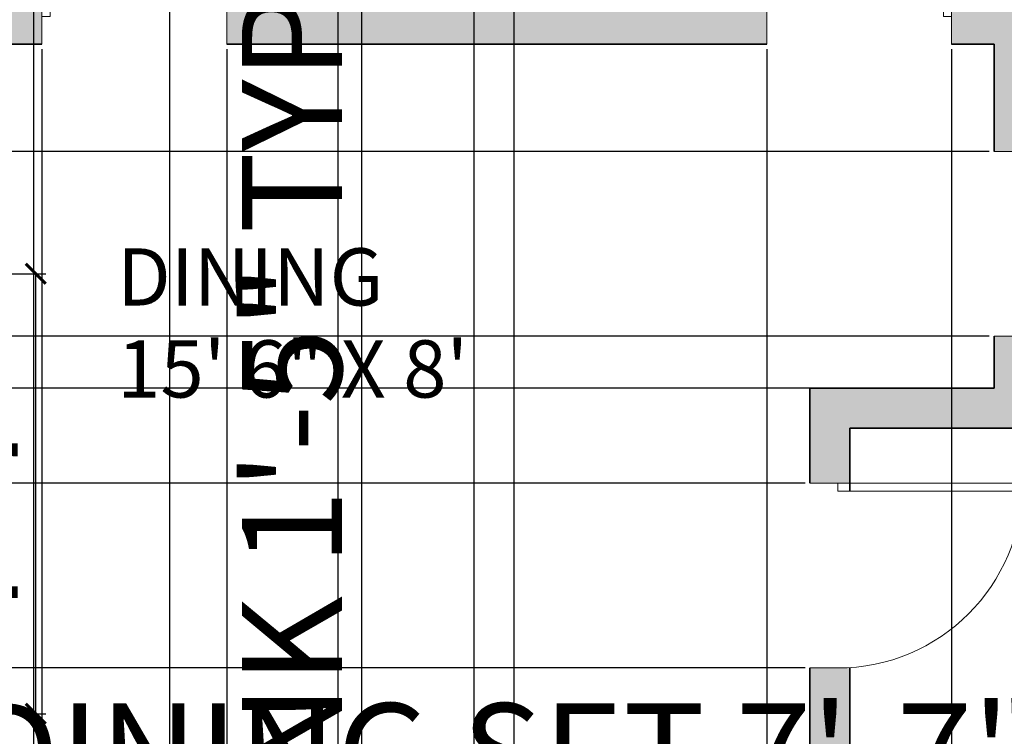
# Model space of a CAD drawing. Units: inches. Extents: x 1763 to 2368, y 1500 to 2097.
# Tile 10 of 24: x 1956 to 2079, y 1794 to 1883. Entities that reach past the tile are written whole.
import ezdxf

# ---------------------------------------------------------------- set-up
doc = ezdxf.new("R2010")
doc.units = ezdxf.units.IN
for name, color, linetype, lineweight in [('A-ANNO-DIMS', 2, 'Continuous', 18), ('A-AREA-IDEN', 7, 'Continuous', 18), ('A-DOOR', 4, 'Continuous', 18), ('A-WALL', 7, 'Continuous', 35), ('A-WALL-PATT', 7, 'Continuous', 13)]:
    doc.layers.add(name, color=color, linetype=linetype, lineweight=lineweight)
doc.styles.get("Standard").update_dxf_attribs({"font": 'arial.ttf'})
doc.dimstyles.new('ISO-25', dxfattribs={"dimtxt": 12.5, "dimasz": 2.5, "dimexe": 1.25, "dimexo": 0.625, "dimtad": 1, "dimdec": 0, "dimlunit": 4, "dimtxsty": 'Standard', "dimblk": 'ARCHTICK', "dimcen": 2.5, "dimclrd": 3, "dimclrt": 4, "dimadec": 0, "dimazin": 0, "dimtfac": 1, "dimtdec": 0, "dimtmove": 0, "dimatfit": 3, "dimfxl": 1, "dimarcsym": 0})

# ---------------------------------------------------------------- blocks, each defined once
blk = doc.blocks.new('*U3')
for p, q in [((0, 0), (0, -6)), ((40, 0), (40, -6))]:
    blk.add_line(p, q)
blk.add_lwpolyline([(0, 0), (0, 40), (1.75, 40), (1.75, 0)], close=True)
blk.add_arc((0, 0), 40, 0, 90)
blk = doc.blocks.new('_ArchTick')
at = {"color": 0, "linetype": 'ByBlock', "const_width": 0.15}
blk.add_lwpolyline([(-0.5, -0.5), (0.5, 0.5)], dxfattribs=at)
blk = doc.blocks.new('*D27')
at = {"layer": 'A-ANNO-DIMS', "color": 0, "lineweight": -2, "transparency": 16777216}
for p, q in [((1853.71, 1795.96), (1853.71, 1781.68)), ((1944.71, 1795.96), (1944.71, 1781.68))]:
    blk.add_line(p, q, dxfattribs=at)
at = {"layer": 'A-ANNO-DIMS', "color": 3, "lineweight": -2, "transparency": 16777216}
for p, q in [((1853.71, 1782.93), (1944.71, 1782.93)), ((1944.71, 1782.93), (2085.85, 1782.93))]:
    blk.add_line(p, q, dxfattribs=at)
at = {"layer": 'Defpoints', "color": 0, "transparency": 16777216}
for p in [(1853.71, 1796.58), (1944.71, 1796.58), (1944.71, 1782.93)]:
    blk.add_point(p, dxfattribs=at)
at = {"layer": 'A-ANNO-DIMS', "color": 3, "lineweight": -2, "transparency": 16777216, "xscale": 2.5, "yscale": 2.5, "zscale": 2.5, "rotation": 180}
blk.add_blockref('_ArchTick', (1853.71, 1782.93), dxfattribs=at)
at = {"layer": 'A-ANNO-DIMS', "color": 3, "lineweight": -2, "transparency": 16777216, "xscale": 2.5, "yscale": 2.5, "zscale": 2.5}
blk.add_blockref('_ArchTick', (1944.71, 1782.93), dxfattribs=at)
at = {"layer": 'A-ANNO-DIMS', "color": 4, "transparency": 16777216, "insert": (2016.53, 1790.02), "char_height": 12.5, "attachment_point": 5}
blk.add_mtext('DINING SET 7\'-7"', dxfattribs=at)
blk = doc.blocks.new('*D28')
at = {"layer": 'A-ANNO-DIMS', "color": 0, "lineweight": -2, "transparency": 16777216}
for p, q in [((1945.34, 1851.58), (1959.61, 1851.58)), ((1945.34, 1796.58), (1959.61, 1796.58))]:
    blk.add_line(p, q, dxfattribs=at)
at = {"layer": 'A-ANNO-DIMS', "color": 3, "lineweight": -2, "transparency": 16777216}
blk.add_line((1958.36, 1796.58), (1958.36, 1851.58), dxfattribs=at)
at = {"layer": 'Defpoints', "color": 0, "transparency": 16777216}
for p in [(1944.71, 1851.58), (1958.36, 1851.58), (1944.71, 1796.58)]:
    blk.add_point(p, dxfattribs=at)
at = {"layer": 'A-ANNO-DIMS', "color": 3, "lineweight": -2, "transparency": 16777216, "xscale": 2.5, "yscale": 2.5, "zscale": 2.5}
for p, rotation in [((1958.36, 1851.58), 90), ((1958.36, 1796.58), 270)]:
    blk.add_blockref('_ArchTick', p, dxfattribs=dict(at, rotation=rotation))
at = {"layer": 'A-ANNO-DIMS', "color": 4, "transparency": 16777216, "insert": (1951.49, 1824.08), "char_height": 12.5, "attachment_point": 5, "rotation": 90}
blk.add_mtext('4\'-7"', dxfattribs=at)
blk = doc.blocks.new('*D33')
at = {"layer": 'A-ANNO-DIMS', "color": 0, "lineweight": -2, "transparency": 16777216}
for p, q in [((2001.02, 1913.28), (1997.82, 1913.28)), ((2001.02, 1896.11), (1997.82, 1896.11))]:
    blk.add_line(p, q, dxfattribs=at)
at = {"layer": 'A-ANNO-DIMS', "color": 3, "lineweight": -2, "transparency": 16777216}
for p, q in [((1999.07, 1913.28), (1999.07, 1896.11)), ((1999.07, 1896.11), (1999.07, 1770.61))]:
    blk.add_line(p, q, dxfattribs=at)
at = {"layer": 'Defpoints', "color": 0, "transparency": 16777216}
for p in [(2001.64, 1913.28), (1999.07, 1896.11), (2001.64, 1896.11)]:
    blk.add_point(p, dxfattribs=at)
at = {"layer": 'A-ANNO-DIMS', "color": 3, "lineweight": -2, "transparency": 16777216, "xscale": 2.5, "yscale": 2.5, "zscale": 2.5}
for p, rotation in [((1999.07, 1913.28), 90), ((1999.07, 1896.11), 270)]:
    blk.add_blockref('_ArchTick', p, dxfattribs=dict(at, rotation=rotation))
at = {"layer": 'A-ANNO-DIMS', "color": 4, "transparency": 16777216, "insert": (1991.98, 1832.11), "char_height": 12.5, "attachment_point": 5, "rotation": 90}
blk.add_mtext('SINK 1\'-5" TYP.', dxfattribs=at)
blk = doc.blocks.new('*D34')
at = {"layer": 'A-ANNO-DIMS', "color": 0, "lineweight": -2, "transparency": 16777216}
for p, q in [((2001.64, 1895.48), (2001.64, 1892.28)), ((2013.09, 1895.48), (2013.09, 1892.28))]:
    blk.add_line(p, q, dxfattribs=at)
at = {"layer": 'A-ANNO-DIMS', "color": 3, "lineweight": -2, "transparency": 16777216}
for p, q in [((2001.64, 1893.53), (2013.09, 1893.53)), ((2013.09, 1893.53), (2131.87, 1893.53))]:
    blk.add_line(p, q, dxfattribs=at)
at = {"layer": 'Defpoints', "color": 0, "transparency": 16777216}
for p in [(2001.64, 1896.11), (2013.09, 1896.11), (2013.09, 1893.53)]:
    blk.add_point(p, dxfattribs=at)
at = {"layer": 'A-ANNO-DIMS', "color": 3, "lineweight": -2, "transparency": 16777216, "xscale": 2.5, "yscale": 2.5, "zscale": 2.5, "rotation": 180}
blk.add_blockref('_ArchTick', (2001.64, 1893.53), dxfattribs=at)
at = {"layer": 'A-ANNO-DIMS', "color": 3, "lineweight": -2, "transparency": 16777216, "xscale": 2.5, "yscale": 2.5, "zscale": 2.5}
blk.add_blockref('_ArchTick', (2013.09, 1893.53), dxfattribs=at)
at = {"layer": 'A-ANNO-DIMS', "color": 4, "transparency": 16777216, "insert": (2073.73, 1900.62), "char_height": 12.5, "attachment_point": 5}
blk.add_mtext('0\'-11 1/2" TYP.', dxfattribs=at)
blk = doc.blocks.new('*D58')
at = {"layer": 'A-ANNO-DIMS', "color": 0, "lineweight": -2, "transparency": 16777216}
for p, q in [((1871.68, 1635.9), (1871.68, 2072.02)), ((1927.07, 1635.9), (1927.07, 2072.02))]:
    blk.add_line(p, q, dxfattribs=at)
at = {"layer": 'A-ANNO-DIMS', "color": 3, "lineweight": -2, "transparency": 16777216}
for p, q in [((1871.68, 2070.77), (1927.07, 2070.77)), ((1927.07, 2070.77), (1993.68, 2070.77))]:
    blk.add_line(p, q, dxfattribs=at)
at = {"layer": 'Defpoints', "color": 0, "transparency": 16777216}
for p in [(1927.07, 2070.77), (1871.68, 1635.27), (1927.07, 1635.27)]:
    blk.add_point(p, dxfattribs=at)
at = {"layer": 'A-ANNO-DIMS', "color": 3, "lineweight": -2, "transparency": 16777216, "xscale": 2.5, "yscale": 2.5, "zscale": 2.5, "rotation": 180}
blk.add_blockref('_ArchTick', (1871.68, 2070.77), dxfattribs=at)
at = {"layer": 'A-ANNO-DIMS', "color": 3, "lineweight": -2, "transparency": 16777216, "xscale": 2.5, "yscale": 2.5, "zscale": 2.5}
blk.add_blockref('_ArchTick', (1927.07, 2070.77), dxfattribs=at)
at = {"layer": 'A-ANNO-DIMS', "color": 4, "transparency": 16777216, "insert": (1961.63, 2077.86), "char_height": 12.5, "attachment_point": 5}
blk.add_mtext('4\'-7 1/2"', dxfattribs=at)
blk = doc.blocks.new('*D68')
at = {"layer": 'A-ANNO-DIMS', "color": 0, "lineweight": -2, "transparency": 16777216}
for p, q in [((1895.59, 1879.65), (1895.59, 1509.91)), ((1932.01, 1879.65), (1932.01, 1509.91))]:
    blk.add_line(p, q, dxfattribs=at)
at = {"layer": 'A-ANNO-DIMS', "color": 3, "lineweight": -2, "transparency": 16777216}
for p, q in [((1895.59, 1511.16), (1932.01, 1511.16)), ((1932.01, 1511.16), (1998.11, 1511.16))]:
    blk.add_line(p, q, dxfattribs=at)
at = {"layer": 'Defpoints', "color": 0, "transparency": 16777216}
for p in [(1895.59, 1880.27), (1932.01, 1880.27), (1932.01, 1511.16)]:
    blk.add_point(p, dxfattribs=at)
at = {"layer": 'A-ANNO-DIMS', "color": 3, "lineweight": -2, "transparency": 16777216, "xscale": 2.5, "yscale": 2.5, "zscale": 2.5, "rotation": 180}
blk.add_blockref('_ArchTick', (1895.59, 1511.16), dxfattribs=at)
at = {"layer": 'A-ANNO-DIMS', "color": 3, "lineweight": -2, "transparency": 16777216, "xscale": 2.5, "yscale": 2.5, "zscale": 2.5}
blk.add_blockref('_ArchTick', (1932.01, 1511.16), dxfattribs=at)
at = {"layer": 'A-ANNO-DIMS', "color": 4, "transparency": 16777216, "insert": (1966.31, 1518.25), "char_height": 12.5, "attachment_point": 5}
blk.add_mtext('3\'-0 1/2"', dxfattribs=at)
blk = doc.blocks.new('*D69')
at = {"layer": 'A-ANNO-DIMS', "color": 0, "lineweight": -2, "transparency": 16777216}
for p, q in [((1838.09, 1879.65), (1838.09, 1509.91)), ((1895.59, 1879.65), (1895.59, 1509.91))]:
    blk.add_line(p, q, dxfattribs=at)
at = {"layer": 'A-ANNO-DIMS', "color": 3, "lineweight": -2, "transparency": 16777216}
for p, q in [((1838.09, 1511.16), (1895.59, 1511.16)), ((1895.59, 1511.16), (1962.2, 1511.16))]:
    blk.add_line(p, q, dxfattribs=at)
at = {"layer": 'Defpoints', "color": 0, "transparency": 16777216}
for p in [(1838.09, 1880.27), (1895.59, 1880.27), (1895.59, 1511.16)]:
    blk.add_point(p, dxfattribs=at)
at = {"layer": 'A-ANNO-DIMS', "color": 3, "lineweight": -2, "transparency": 16777216, "xscale": 2.5, "yscale": 2.5, "zscale": 2.5, "rotation": 180}
blk.add_blockref('_ArchTick', (1838.09, 1511.16), dxfattribs=at)
at = {"layer": 'A-ANNO-DIMS', "color": 3, "lineweight": -2, "transparency": 16777216, "xscale": 2.5, "yscale": 2.5, "zscale": 2.5}
blk.add_blockref('_ArchTick', (1895.59, 1511.16), dxfattribs=at)
at = {"layer": 'A-ANNO-DIMS', "color": 4, "transparency": 16777216, "insert": (1930.15, 1518.24), "char_height": 12.5, "attachment_point": 5}
blk.add_mtext('4\'-9 1/2"', dxfattribs=at)
blk = doc.blocks.new('*D70')
at = {"layer": 'A-ANNO-DIMS', "color": 0, "lineweight": -2, "transparency": 16777216}
for p, q in [((1959.13, 1879.65), (1959.13, 1509.91)), ((1982.23, 1879.65), (1982.23, 1509.91))]:
    blk.add_line(p, q, dxfattribs=at)
at = {"layer": 'A-ANNO-DIMS', "color": 3, "lineweight": -2, "transparency": 16777216}
for p, q in [((1959.13, 1511.16), (1982.23, 1511.16)), ((1982.23, 1511.16), (2027.75, 1511.16))]:
    blk.add_line(p, q, dxfattribs=at)
at = {"layer": 'Defpoints', "color": 0, "transparency": 16777216}
for p in [(1959.13, 1880.27), (1982.23, 1880.27), (1982.23, 1511.16)]:
    blk.add_point(p, dxfattribs=at)
at = {"layer": 'A-ANNO-DIMS', "color": 3, "lineweight": -2, "transparency": 16777216, "xscale": 2.5, "yscale": 2.5, "zscale": 2.5, "rotation": 180}
blk.add_blockref('_ArchTick', (1959.13, 1511.16), dxfattribs=at)
at = {"layer": 'A-ANNO-DIMS', "color": 3, "lineweight": -2, "transparency": 16777216, "xscale": 2.5, "yscale": 2.5, "zscale": 2.5}
blk.add_blockref('_ArchTick', (1982.23, 1511.16), dxfattribs=at)
at = {"layer": 'A-ANNO-DIMS', "color": 4, "transparency": 16777216, "insert": (2006.24, 1518.06), "char_height": 12.5, "attachment_point": 5}
blk.add_mtext('1\'-11"', dxfattribs=at)
blk = doc.blocks.new('*D71')
at = {"layer": 'A-ANNO-DIMS', "color": 0, "lineweight": -2, "transparency": 16777216}
for p, q in [((2049.69, 1879.65), (2049.69, 1509.91)), ((2072.78, 1879.65), (2072.78, 1509.91))]:
    blk.add_line(p, q, dxfattribs=at)
at = {"layer": 'A-ANNO-DIMS', "color": 3, "lineweight": -2, "transparency": 16777216}
for p, q in [((2049.69, 1511.16), (2072.78, 1511.16)), ((2072.78, 1511.16), (2118.3, 1511.16))]:
    blk.add_line(p, q, dxfattribs=at)
at = {"layer": 'Defpoints', "color": 0, "transparency": 16777216}
for p in [(2049.69, 1880.27), (2072.78, 1880.27), (2072.78, 1511.16)]:
    blk.add_point(p, dxfattribs=at)
at = {"layer": 'A-ANNO-DIMS', "color": 3, "lineweight": -2, "transparency": 16777216, "xscale": 2.5, "yscale": 2.5, "zscale": 2.5, "rotation": 180}
blk.add_blockref('_ArchTick', (2049.69, 1511.16), dxfattribs=at)
at = {"layer": 'A-ANNO-DIMS', "color": 3, "lineweight": -2, "transparency": 16777216, "xscale": 2.5, "yscale": 2.5, "zscale": 2.5}
blk.add_blockref('_ArchTick', (2072.78, 1511.16), dxfattribs=at)
at = {"layer": 'A-ANNO-DIMS', "color": 4, "transparency": 16777216, "insert": (2096.79, 1518.06), "char_height": 12.5, "attachment_point": 5}
blk.add_mtext('1\'-11"', dxfattribs=at)
blk = doc.blocks.new('*D77')
at = {"layer": 'A-ANNO-DIMS', "color": 0, "lineweight": -2, "transparency": 16777216}
for p, q in [((1975.09, 1972.65), (1975.09, 1509.91)), ((1996.09, 1972.65), (1996.09, 1509.91))]:
    blk.add_line(p, q, dxfattribs=at)
at = {"layer": 'A-ANNO-DIMS', "color": 3, "lineweight": -2, "transparency": 16777216}
for p, q in [((1975.09, 1511.16), (1996.09, 1511.16)), ((1996.09, 1511.16), (2031.89, 1511.16))]:
    blk.add_line(p, q, dxfattribs=at)
at = {"layer": 'Defpoints', "color": 0, "transparency": 16777216}
for p in [(1975.09, 1973.27), (1996.09, 1973.27), (1996.09, 1511.16)]:
    blk.add_point(p, dxfattribs=at)
at = {"layer": 'A-ANNO-DIMS', "color": 3, "lineweight": -2, "transparency": 16777216, "xscale": 2.5, "yscale": 2.5, "zscale": 2.5, "rotation": 180}
blk.add_blockref('_ArchTick', (1975.09, 1511.16), dxfattribs=at)
at = {"layer": 'A-ANNO-DIMS', "color": 3, "lineweight": -2, "transparency": 16777216, "xscale": 2.5, "yscale": 2.5, "zscale": 2.5}
blk.add_blockref('_ArchTick', (1996.09, 1511.16), dxfattribs=at)
at = {"layer": 'A-ANNO-DIMS', "color": 4, "transparency": 16777216, "insert": (2015.24, 1518.16), "char_height": 12.5, "attachment_point": 5}
blk.add_mtext('1\'-9"', dxfattribs=at)
blk = doc.blocks.new('*D79')
at = {"layer": 'A-ANNO-DIMS', "color": 3, "lineweight": -2, "transparency": 16777216}
for p, q in [((1788.85, 1825.4), (1788.85, 1870.91)), ((1788.85, 1802.3), (1788.85, 1825.4))]:
    blk.add_line(p, q, dxfattribs=at)
at = {"layer": 'A-ANNO-DIMS', "color": 0, "lineweight": -2, "transparency": 16777216}
for p, q in [((2054.47, 1825.4), (1787.6, 1825.4)), ((2054.47, 1802.3), (1787.6, 1802.3))]:
    blk.add_line(p, q, dxfattribs=at)
at = {"layer": 'Defpoints', "color": 0, "transparency": 16777216}
for p in [(1788.85, 1825.4), (2055.09, 1825.4), (2055.09, 1802.3)]:
    blk.add_point(p, dxfattribs=at)
at = {"layer": 'A-ANNO-DIMS', "color": 3, "lineweight": -2, "transparency": 16777216, "xscale": 2.5, "yscale": 2.5, "zscale": 2.5}
for p, rotation in [((1788.85, 1825.4), 90), ((1788.85, 1802.3), 270)]:
    blk.add_blockref('_ArchTick', p, dxfattribs=dict(at, rotation=rotation))
at = {"layer": 'A-ANNO-DIMS', "color": 4, "transparency": 16777216, "insert": (1781.95, 1849.4), "char_height": 12.5, "attachment_point": 5, "rotation": 90}
blk.add_mtext('1\'-11"', dxfattribs=at)
blk = doc.blocks.new('*D80')
at = {"layer": 'A-ANNO-DIMS', "color": 3, "lineweight": -2, "transparency": 16777216}
for p, q in [((1788.85, 1837.27), (1788.85, 1873.07)), ((1788.85, 1825.4), (1788.85, 1837.27))]:
    blk.add_line(p, q, dxfattribs=at)
at = {"layer": 'A-ANNO-DIMS', "color": 0, "lineweight": -2, "transparency": 16777216}
for p, q in [((2054.47, 1837.27), (1787.6, 1837.27)), ((2054.47, 1825.4), (1787.6, 1825.4))]:
    blk.add_line(p, q, dxfattribs=at)
at = {"layer": 'Defpoints', "color": 0, "transparency": 16777216}
for p in [(1788.85, 1837.27), (2055.09, 1837.27), (2055.09, 1825.4)]:
    blk.add_point(p, dxfattribs=at)
at = {"layer": 'A-ANNO-DIMS', "color": 3, "lineweight": -2, "transparency": 16777216, "xscale": 2.5, "yscale": 2.5, "zscale": 2.5}
for p, rotation in [((1788.85, 1837.27), 90), ((1788.85, 1825.4), 270)]:
    blk.add_blockref('_ArchTick', p, dxfattribs=dict(at, rotation=rotation))
at = {"layer": 'A-ANNO-DIMS', "color": 4, "transparency": 16777216, "insert": (1781.85, 1856.42), "char_height": 12.5, "attachment_point": 5, "rotation": 90}
blk.add_mtext('1\'-0"', dxfattribs=at)
blk = doc.blocks.new('*D81')
at = {"layer": 'A-ANNO-DIMS', "color": 3, "lineweight": -2, "transparency": 16777216}
for p, q in [((1788.85, 1866.87), (1788.85, 1912.38)), ((1788.85, 1843.77), (1788.85, 1866.87))]:
    blk.add_line(p, q, dxfattribs=at)
at = {"layer": 'A-ANNO-DIMS', "color": 0, "lineweight": -2, "transparency": 16777216}
for p, q in [((2077.47, 1866.87), (1787.6, 1866.87)), ((2077.47, 1843.77), (1787.6, 1843.77))]:
    blk.add_line(p, q, dxfattribs=at)
at = {"layer": 'Defpoints', "color": 0, "transparency": 16777216}
for p in [(1788.85, 1866.87), (2078.09, 1866.87), (2078.09, 1843.77)]:
    blk.add_point(p, dxfattribs=at)
at = {"layer": 'A-ANNO-DIMS', "color": 3, "lineweight": -2, "transparency": 16777216, "xscale": 2.5, "yscale": 2.5, "zscale": 2.5}
for p, rotation in [((1788.85, 1866.87), 90), ((1788.85, 1843.77), 270)]:
    blk.add_blockref('_ArchTick', p, dxfattribs=dict(at, rotation=rotation))
at = {"layer": 'A-ANNO-DIMS', "color": 4, "transparency": 16777216, "insert": (1781.95, 1890.87), "char_height": 12.5, "attachment_point": 5, "rotation": 90}
blk.add_mtext('1\'-11"', dxfattribs=at)
blk = doc.blocks.new('*D82')
at = {"layer": 'A-ANNO-DIMS', "color": 3, "lineweight": -2, "transparency": 16777216}
for p, q in [((1788.85, 1843.77), (1788.85, 1909.87)), ((1788.85, 1837.27), (1788.85, 1843.77))]:
    blk.add_line(p, q, dxfattribs=at)
at = {"layer": 'A-ANNO-DIMS', "color": 0, "lineweight": -2, "transparency": 16777216}
for p, q in [((2077.47, 1843.77), (1787.6, 1843.77)), ((2077.47, 1837.27), (1787.6, 1837.27))]:
    blk.add_line(p, q, dxfattribs=at)
at = {"layer": 'Defpoints', "color": 0, "transparency": 16777216}
for p in [(1788.85, 1843.77), (2078.09, 1843.77), (2078.09, 1837.27)]:
    blk.add_point(p, dxfattribs=at)
at = {"layer": 'A-ANNO-DIMS', "color": 3, "lineweight": -2, "transparency": 16777216, "xscale": 2.5, "yscale": 2.5, "zscale": 2.5}
for p, rotation in [((1788.85, 1843.77), 90), ((1788.85, 1837.27), 270)]:
    blk.add_blockref('_ArchTick', p, dxfattribs=dict(at, rotation=rotation))
at = {"layer": 'A-ANNO-DIMS', "color": 4, "transparency": 16777216, "insert": (1781.77, 1878.07), "char_height": 12.5, "attachment_point": 5, "rotation": 90}
blk.add_mtext('0\'-6 1/2"', dxfattribs=at)
blk = doc.blocks.new('*D85')
at = {"layer": 'A-ANNO-DIMS', "color": 0, "lineweight": -2, "transparency": 16777216}
for p, q in [((1957.47, 1986.27), (1787.6, 1986.27)), ((1958.51, 1880.27), (1787.6, 1880.27))]:
    blk.add_line(p, q, dxfattribs=at)
at = {"layer": 'A-ANNO-DIMS', "color": 3, "lineweight": -2, "transparency": 16777216}
blk.add_line((1788.85, 1986.27), (1788.85, 1880.27), dxfattribs=at)
at = {"layer": 'Defpoints', "color": 0, "transparency": 16777216}
for p in [(1958.09, 1986.27), (1788.85, 1880.27), (1959.13, 1880.27)]:
    blk.add_point(p, dxfattribs=at)
at = {"layer": 'A-ANNO-DIMS', "color": 3, "lineweight": -2, "transparency": 16777216, "xscale": 2.5, "yscale": 2.5, "zscale": 2.5}
for p, rotation in [((1788.85, 1986.27), 90), ((1788.85, 1880.27), 270)]:
    blk.add_blockref('_ArchTick', p, dxfattribs=dict(at, rotation=rotation))
at = {"layer": 'A-ANNO-DIMS', "color": 4, "transparency": 16777216, "insert": (1781.85, 1933.27), "char_height": 12.5, "attachment_point": 5, "rotation": 90}
blk.add_mtext('8\'-10"', dxfattribs=at)
blk = doc.blocks.new('*D86')
at = {"layer": 'A-ANNO-DIMS', "color": 0, "lineweight": -2, "transparency": 16777216}
for p, q in [((2013.09, 1884.65), (2013.09, 1509.91)), ((2018.09, 1884.65), (2018.09, 1509.91))]:
    blk.add_line(p, q, dxfattribs=at)
at = {"layer": 'A-ANNO-DIMS', "color": 3, "lineweight": -2, "transparency": 16777216}
for p, q in [((2013.09, 1511.16), (2018.09, 1511.16)), ((2018.09, 1511.16), (2055.07, 1511.16))]:
    blk.add_line(p, q, dxfattribs=at)
at = {"layer": 'Defpoints', "color": 0, "transparency": 16777216}
for p in [(2013.09, 1885.27), (2018.09, 1885.27), (2018.09, 1511.16)]:
    blk.add_point(p, dxfattribs=at)
at = {"layer": 'A-ANNO-DIMS', "color": 3, "lineweight": -2, "transparency": 16777216, "xscale": 2.5, "yscale": 2.5, "zscale": 2.5, "rotation": 180}
blk.add_blockref('_ArchTick', (2013.09, 1511.16), dxfattribs=at)
at = {"layer": 'A-ANNO-DIMS', "color": 3, "lineweight": -2, "transparency": 16777216, "xscale": 2.5, "yscale": 2.5, "zscale": 2.5}
blk.add_blockref('_ArchTick', (2018.09, 1511.16), dxfattribs=at)
at = {"layer": 'A-ANNO-DIMS', "color": 4, "transparency": 16777216, "insert": (2037.83, 1518.16), "char_height": 12.5, "attachment_point": 5}
blk.add_mtext('0\'-5"', dxfattribs=at)
blk = doc.blocks.new('*D87')
at = {"layer": 'A-ANNO-DIMS', "color": 0, "lineweight": -2, "transparency": 16777216}
for p, q in [((1958.09, 1980.65), (1958.09, 1509.91)), ((1975.09, 1980.65), (1975.09, 1509.91))]:
    blk.add_line(p, q, dxfattribs=at)
at = {"layer": 'A-ANNO-DIMS', "color": 3, "lineweight": -2, "transparency": 16777216}
for p, q in [((1958.09, 1511.16), (1975.09, 1511.16)), ((1975.09, 1511.16), (2010.89, 1511.16))]:
    blk.add_line(p, q, dxfattribs=at)
at = {"layer": 'Defpoints', "color": 0, "transparency": 16777216}
for p in [(1958.09, 1981.27), (1975.09, 1981.27), (1975.09, 1511.16)]:
    blk.add_point(p, dxfattribs=at)
at = {"layer": 'A-ANNO-DIMS', "color": 3, "lineweight": -2, "transparency": 16777216, "xscale": 2.5, "yscale": 2.5, "zscale": 2.5, "rotation": 180}
blk.add_blockref('_ArchTick', (1958.09, 1511.16), dxfattribs=at)
at = {"layer": 'A-ANNO-DIMS', "color": 3, "lineweight": -2, "transparency": 16777216, "xscale": 2.5, "yscale": 2.5, "zscale": 2.5}
blk.add_blockref('_ArchTick', (1975.09, 1511.16), dxfattribs=at)
at = {"layer": 'A-ANNO-DIMS', "color": 4, "transparency": 16777216, "insert": (1994.24, 1518.16), "char_height": 12.5, "attachment_point": 5}
blk.add_mtext('1\'-5"', dxfattribs=at)

msp = doc.modelspace()

# ---------------------------------------------------------------- hatches: boundary and pattern name
at = {"layer": 'A-WALL-PATT'}
h = msp.add_hatch(color=256, dxfattribs=at)
h.dxf.hatch_style = 1
h.paths.add_polyline_path([(1838.09, 2034.27), (1838.09, 2043.27), (1829.09, 2043.27), (1829.09, 1953.39), (1838.09, 1953.39)])
h.paths.add_polyline_path([(1838.09, 1913.1), (1829.09, 1913.1), (1829.09, 1862.2), (1838.09, 1862.2)])
h.paths.add_polyline_path([(1838.09, 1825.59), (1829.09, 1825.59), (1829.09, 1738.64), (1838.09, 1738.64)])
h.paths.add_polyline_path([(1895.59, 1885.27), (1838.09, 1885.27), (1838.09, 1880.27), (1895.59, 1880.27)])
h.paths.add_polyline_path([(1857.39, 1784.27), (1838.09, 1784.27), (1838.09, 1779.27), (1857.39, 1779.27)])
h.paths.add_polyline_path([(1958.09, 1981.27), (1971.46, 1981.27), (1971.46, 1986.27), (1968.57, 1986.27), (1958.09, 1986.27), (1953.09, 1986.27), (1927.39, 1986.27), (1927.39, 1981.27), (1953.09, 1981.27), (1953.09, 1885.27), (1932.01, 1885.27), (1932.01, 1880.27), (1959.13, 1880.27), (1959.13, 1883.74), (1959.13, 1885.27), (1958.09, 1885.27)])
h.paths.add_polyline_path([(2018.09, 1981.27), (2031.02, 1981.27), (2031.02, 1986.27), (2018.09, 1986.27), (2013.09, 1986.27), (2001.23, 1986.27), (2001.23, 1981.27), (2013.09, 1981.27), (2013.09, 1885.27), (1982.18, 1885.27, -0.016629), (1982.23, 1883.74), (1982.23, 1880.27), (2049.69, 1880.27), (2049.69, 1883.74, -0.016629), (2049.74, 1885.27), (2018.09, 1885.27)])
h.paths.add_polyline_path([(2083.09, 1981.27), (2120.61, 1981.27), (2120.61, 1986.27), (2083.09, 1986.27), (2078.09, 1986.27), (2063.14, 1986.27), (2063.14, 1981.27), (2078.09, 1981.27), (2078.09, 1885.27), (2072.78, 1885.27), (2072.78, 1883.74), (2072.78, 1880.27), (2078.09, 1880.27), (2078.09, 1866.87), (2081.56, 1866.87, -0.016629), (2083.09, 1866.82)])
h.paths.add_polyline_path([(1871.68, 1635.27), (1838.09, 1635.27), (1838.09, 1626.27), (1871.68, 1626.27)], flags=17)
h.paths.add_polyline_path([(2100.58, 1688.27), (2060.09, 1688.27), (2060.09, 1679.27), (2100.58, 1679.27)], flags=17)
h.paths.add_polyline_path([(2180.09, 1688.27), (2148.74, 1688.27), (2148.74, 1679.27), (2180.09, 1679.27)], flags=17)
h.paths.add_polyline_path([(2189.09, 1746.22), (2180.09, 1746.22), (2180.09, 1743.42), (2180.12, 1743.42), (2180.12, 1726.72), (2180.09, 1572.27), (2034.91, 1572.27), (2034.91, 1565.6), (2034.91, 1563.27), (2189.09, 1563.27)])
h.paths.add_polyline_path([(2060.09, 1802.35, -0.016629), (2058.56, 1802.3), (2055.09, 1802.3), (2055.09, 1635.27), (2042.48, 1635.27), (2042.48, 1629.74), (2042.48, 1626.27), (2055.09, 1626.27), (2055.09, 1599.27), (2040.27, 1599.27), (2040.27, 1590.27), (2060.09, 1590.27)])
h.paths.add_polyline_path([(2019.39, 1629.74, -0.060569), (2020.06, 1635.27), (1995.09, 1635.27), (1990.09, 1635.27), (1927.07, 1635.27), (1927.07, 1626.27), (1990.09, 1626.27), (1990.09, 1590.27), (1995.09, 1590.27), (2005.2, 1590.27), (2005.2, 1599.27), (1995.09, 1599.27), (1995.09, 1626.27), (2019.39, 1626.27)])
edge = h.paths.add_edge_path()
edge.add_line((2180.09, 1837.27), (2167.2, 1837.27))
edge.add_spline(control_points=[(2167.2, 1837.27), (2167.19, 1837.27), (2167.18, 1837.27), (2167.18, 1837.27)], knot_values=[168.955493, 168.955493, 168.955493, 168.955493, 169.065871, 169.065871, 169.065871, 169.065871], degree=3, periodic=0)
edge.add_spline(control_points=[(2167.18, 1837.27), (2166.56, 1837.38), (2166.33, 1846.16), (2165.71, 1846.24)], knot_values=[159.864705, 159.864705, 159.864705, 159.864705, 168.955493, 168.955493, 168.955493, 168.955493], degree=3, periodic=0)
edge.add_line((2167.12, 1837.27), (2163.16, 1837.27))
edge.add_spline(control_points=[(2163.16, 1837.27), (2163.16, 1837.27), (2163.16, 1837.27), (2163.15, 1837.27)], knot_values=[150.537172, 150.537172, 150.537172, 150.537172, 150.553797, 150.553797, 150.553797, 150.553797], degree=3, periodic=0)
edge.add_spline(control_points=[(2163.15, 1837.27), (2162.29, 1837.29), (2161.59, 1846.23), (2160.88, 1846.24)], knot_values=[141.293426, 141.293426, 141.293426, 141.293426, 150.537172, 150.537172, 150.537172, 150.537172], degree=3, periodic=0)
edge.add_line((2163.08, 1837.27), (2158.7, 1837.27))
edge.add_spline(control_points=[(2158.7, 1837.27), (2158.7, 1837.27), (2158.7, 1837.27), (2158.7, 1837.27)], knot_values=[132.033544, 132.033544, 132.033544, 132.033544, 132.049151, 132.049151, 132.049151, 132.049151], degree=3, periodic=0)
edge.add_spline(control_points=[(2158.7, 1837.27), (2157.97, 1837.29), (2157.26, 1846.23), (2156.39, 1846.24)], knot_values=[122.786021, 122.786021, 122.786021, 122.786021, 132.033544, 132.033544, 132.033544, 132.033544], degree=3, periodic=0)
edge.add_line((2158.63, 1837.27), (2153.84, 1837.27))
edge.add_spline(control_points=[(2153.84, 1837.27), (2153.83, 1837.27), (2153.82, 1837.27), (2153.82, 1837.27)], knot_values=[113.451585, 113.451585, 113.451585, 113.451585, 113.562103, 113.562103, 113.562103, 113.562103], degree=3, periodic=0)
edge.add_spline(control_points=[(2153.82, 1837.27), (2153.17, 1837.38), (2152.88, 1846.19), (2152.4, 1846.24)], knot_values=[0, 0, 0, 0, 9.081854, 9.081854, 9.081854, 9.081854], degree=3, periodic=0)
edge.add_line((2153.76, 1837.27), (2150.39, 1837.27))
edge.add_spline(control_points=[(2150.39, 1837.27), (2150.38, 1837.27), (2150.37, 1837.27), (2150.36, 1837.27)], knot_values=[95.069382, 95.069382, 95.069382, 95.069382, 95.17519, 95.17519, 95.17519, 95.17519], degree=3, periodic=0)
edge.add_spline(control_points=[(2150.36, 1837.27), (2149.49, 1837.37), (2148.42, 1846.19), (2147.59, 1846.24)], knot_values=[85.824599, 85.824599, 85.824599, 85.824599, 95.069382, 95.069382, 95.069382, 95.069382], degree=3, periodic=0)
edge.add_line((2150.29, 1837.27), (2145.43, 1837.27))
edge.add_spline(control_points=[(2145.43, 1837.27), (2145.43, 1837.27), (2145.42, 1837.27), (2145.42, 1837.27)], knot_values=[76.505559, 76.505559, 76.505559, 76.505559, 76.547811, 76.547811, 76.547811, 76.547811], degree=3, periodic=0)
edge.add_spline(control_points=[(2145.42, 1837.27), (2144.68, 1837.31), (2143.8, 1846.19), (2142.95, 1846.24)], knot_values=[67.23945, 67.23945, 67.23945, 67.23945, 76.505559, 76.505559, 76.505559, 76.505559], degree=3, periodic=0)
edge.add_line((2145.35, 1837.27), (2134.57, 1837.27))
edge.add_spline(control_points=[(2134.57, 1837.27), (2134.57, 1837.27), (2134.56, 1837.27), (2134.56, 1837.27)], knot_values=[39.001463, 39.001463, 39.001463, 39.001463, 39.045107, 39.045107, 39.045107, 39.045107], degree=3, periodic=0)
edge.add_spline(control_points=[(2134.56, 1837.27), (2133.87, 1837.31), (2133.4, 1845.85), (2132.33, 1846.24)], knot_values=[29.79778, 29.79778, 29.79778, 29.79778, 39.001463, 39.001463, 39.001463, 39.001463], degree=3, periodic=0)
edge.add_line((2134.5, 1837.27), (2128.08, 1837.27))
edge.add_spline(control_points=[(2128.08, 1837.27), (2128.03, 1837.26), (2127.98, 1837.26), (2127.93, 1837.27)], knot_values=[19.482067, 19.482067, 19.482067, 19.482067, 19.869396, 19.869396, 19.869396, 19.869396], degree=3, periodic=0)
edge.add_spline(control_points=[(2125.01, 1846.24), (2126.16, 1844.66), (2126.82, 1837.57), (2127.93, 1837.27)], knot_values=[10.389805, 10.389805, 10.389805, 10.389805, 19.482067, 19.482067, 19.482067, 19.482067], degree=3, periodic=0)
edge.add_line((2127.93, 1837.27), (2083.09, 1837.27))
edge.add_line((2083.09, 1837.27), (2083.09, 1843.77))
edge.add_line((2083.09, 1843.77), (2081.56, 1843.77))
edge.add_line((2081.56, 1843.77), (2078.09, 1843.77))
edge.add_line((2078.09, 1843.77), (2078.09, 1837.27))
edge.add_line((2078.09, 1837.27), (2055.09, 1837.27))
edge.add_line((2055.09, 1837.27), (2055.09, 1825.4))
edge.add_line((2055.09, 1825.4), (2058.56, 1825.4))
edge.add_line((2058.56, 1825.4), (2060.09, 1825.4))
edge.add_line((2060.09, 1825.4), (2060.09, 1832.27))
edge.add_line((2060.09, 1832.27), (2122.44, 1832.27))
edge.add_spline(control_points=[(2122.44, 1832.27), (2122.73, 1832.58), (2123.01, 1832.62), (2123.28, 1832.27)], knot_values=[5.972033, 5.972033, 5.972033, 5.972033, 8.057258, 8.057258, 8.057258, 8.057258], degree=3, periodic=0)
edge.add_line((2123.28, 1832.27), (2137.95, 1832.27))
edge.add_spline(control_points=[(2137.95, 1832.27), (2137.96, 1832.27), (2137.97, 1832.27), (2137.98, 1832.27)], knot_values=[53.926862, 53.926862, 53.926862, 53.926862, 54.030075, 54.030075, 54.030075, 54.030075], degree=3, periodic=0)
edge.add_spline(control_points=[(2139.72, 1825.02), (2139.28, 1825.06), (2138.67, 1832.18), (2137.98, 1832.27)], knot_values=[54.030075, 54.030075, 54.030075, 54.030075, 61.445194, 61.445194, 61.445194, 61.445194], degree=3, periodic=0)
edge.add_line((2138.05, 1832.27), (2140.96, 1832.27))
edge.add_spline(control_points=[(2140.96, 1832.27), (2140.97, 1832.27), (2140.98, 1832.27), (2140.99, 1832.27)], knot_values=[68.854182, 68.854182, 68.854182, 68.854182, 68.971237, 68.971237, 68.971237, 68.971237], degree=3, periodic=0)
edge.add_spline(control_points=[(2143.19, 1825.02), (2142.44, 1825.07), (2141.56, 1832.16), (2140.99, 1832.27)], knot_values=[68.971237, 68.971237, 68.971237, 68.971237, 76.444911, 76.444911, 76.444911, 76.444911], degree=3, periodic=0)
edge.add_line((2141.04, 1832.27), (2145.43, 1832.27))
edge.add_spline(control_points=[(2145.43, 1832.27), (2145.44, 1832.27), (2145.45, 1832.27), (2145.46, 1832.27)], knot_values=[84.039047, 84.039047, 84.039047, 84.039047, 84.124041, 84.124041, 84.124041, 84.124041], degree=3, periodic=0)
edge.add_spline(control_points=[(2148.11, 1825.02), (2147.34, 1825.02), (2146.3, 1832.19), (2145.46, 1832.27)], knot_values=[84.124041, 84.124041, 84.124041, 84.124041, 91.773891, 91.773891, 91.773891, 91.773891], degree=3, periodic=0)
edge.add_line((2145.54, 1832.27), (2150.39, 1832.27))
edge.add_spline(control_points=[(2150.39, 1832.27), (2150.42, 1832.28), (2150.45, 1832.28), (2150.47, 1832.27)], knot_values=[99.381577, 99.381577, 99.381577, 99.381577, 99.573457, 99.573457, 99.573457, 99.573457], degree=3, periodic=0)
edge.add_spline(control_points=[(2153.97, 1825.02), (2153.09, 1825.28), (2151.53, 1832.1), (2150.47, 1832.27)], knot_values=[99.573457, 99.573457, 99.573457, 99.573457, 107.218357, 107.218357, 107.218357, 107.218357], degree=3, periodic=0)
edge.add_line((2150.57, 1832.27), (2155.6, 1832.27))
edge.add_spline(control_points=[(2155.6, 1832.27), (2155.6, 1832.27), (2155.61, 1832.27), (2155.62, 1832.27)], knot_values=[114.933058, 114.933058, 114.933058, 114.933058, 115.013624, 115.013624, 115.013624, 115.013624], degree=3, periodic=0)
edge.add_spline(control_points=[(2158.28, 1825.02), (2157.4, 1825.07), (2156.25, 1832.2), (2155.62, 1832.27)], knot_values=[115.013624, 115.013624, 115.013624, 115.013624, 122.616269, 122.616269, 122.616269, 122.616269], degree=3, periodic=0)
edge.add_line((2155.68, 1832.27), (2165.19, 1832.27))
edge.add_spline(control_points=[(2165.19, 1832.27), (2165.2, 1832.27), (2165.2, 1832.27), (2165.2, 1832.27)], knot_values=[145.488477, 145.488477, 145.488477, 145.488477, 145.516379, 145.516379, 145.516379, 145.516379], degree=3, periodic=0)
edge.add_spline(control_points=[(2167.45, 1825.02), (2166.96, 1825.02), (2166.06, 1832.25), (2165.2, 1832.27)], knot_values=[145.516379, 145.516379, 145.516379, 145.516379, 153.105469, 153.105469, 153.105469, 153.105469], degree=3, periodic=0)
edge.add_line((2165.29, 1832.27), (2168.93, 1832.27))
edge.add_spline(control_points=[(2168.93, 1832.27), (2168.98, 1832.29), (2169.04, 1832.29), (2169.1, 1832.27)], knot_values=[160.517439, 160.517439, 160.517439, 160.517439, 160.939723, 160.939723, 160.939723, 160.939723], degree=3, periodic=0)
edge.add_spline(control_points=[(2171.09, 1828.64), (2170.35, 1830.37), (2169.62, 1832.09), (2169.1, 1832.27)], knot_values=[160.939723, 160.939723, 160.939723, 160.939723, 164.738835, 164.738835, 164.738835, 164.738835], degree=3, periodic=0)
edge.add_line((2169.1, 1832.27), (2180.09, 1832.27))
edge.add_line((2180.09, 1832.27), (2180.09, 1837.27))
h.paths.add_polyline_path([(2189.09, 1885.52), (2180.09, 1885.52), (2180.09, 1813.32), (2180.12, 1813.32), (2180.12, 1796.62), (2180.12, 1795.26), (2189.09, 1795.26)])
h.paths.add_polyline_path([(2180.09, 1986.27), (2166.28, 1986.27), (2166.28, 1981.27), (2180.09, 1981.27)])
h.paths.add_polyline_path([(2189.09, 2043.27), (2180.09, 2043.27), (2180.09, 2034.27), (2180.09, 1934.11), (2189.09, 1934.11)])
h.paths.add_polyline_path([(1838.09, 1681.59), (1829.09, 1681.59), (1829.09, 1563.27), (2003.86, 1563.27), (2003.86, 1565.6), (2003.86, 1572.27), (1838.09, 1572.27)])

# ---------------------------------------------------------------- linework, layer by layer
at = {"layer": 'A-WALL'}
for p, q in [((1932.01, 1880.27), (1959.13, 1880.27)), ((1982.23, 1880.27), (2049.69, 1880.27)), ((2072.78, 1880.27), (2078.09, 1880.27)), ((2078.09, 1866.87), (2078.09, 1880.27)), ((2078.09, 1837.27), (2078.09, 1843.77)), ((2055.09, 1837.27), (2078.09, 1837.27)), ((2055.09, 1837.27), (2055.09, 1825.4)), ((2060.09, 1832.27), (2180.09, 1832.27)), ((2060.09, 1832.27), (2060.09, 1824.38)), ((2055.09, 1802.3), (2055.09, 1635.27)), ((2060.09, 1802.35), (2060.09, 1590.27))]:
    msp.add_line(p, q, dxfattribs=at)

# ---------------------------------------------------------------- block references
at = {"layer": 'A-DOOR', "yscale": 0.5774759422388936, "zscale": 0.5774759422388936}
for p, xscale in [((1959.13, 1883.74), 0.5774759422388936), ((2072.78, 1883.74), -0.5774759422388936)]:
    msp.add_blockref('*U3', p, dxfattribs=dict(at, xscale=xscale))
at = {"layer": 'A-DOOR', "yscale": 0.5774759422388936, "zscale": 0.5774759422388936, "rotation": 270}
for p, xscale in [((2081.56, 1843.77), -0.5774759422388936), ((2058.56, 1825.4), 0.5774759422388936)]:
    msp.add_blockref('*U3', p, dxfattribs=dict(at, xscale=xscale))

# ---------------------------------------------------------------- texts
at = {"layer": 'A-AREA-IDEN'}
for s, height, p in [('DINING', 7.155, (1968.52, 1847.61)), ('15\' 6" X 8\'', 7.1545, (1968.52, 1836.11))]:
    msp.add_text(s, height=height, dxfattribs=at).set_placement(p)

# ---------------------------------------------------------------- dimensions: what is measured, and where the dimension line sits
at = {"layer": 'A-ANNO-DIMS'}
for base, p1, p2, picture, middle in [((1927.07, 2070.77), (1871.68, 1635.27), (1927.07, 1635.27), '*D58', (1961.63, 2077.86)), ((1975.09, 1511.16), (1958.09, 1981.27), (1975.09, 1981.27), '*D87', (1994.24, 1518.16)), ((1996.09, 1511.16), (1975.09, 1973.27), (1996.09, 1973.27), '*D77', (2015.24, 1518.16)), ((2018.09, 1511.16), (2013.09, 1885.27), (2018.09, 1885.27), '*D86', (2037.83, 1518.16)), ((1895.59, 1511.16), (1838.09, 1880.27), (1895.59, 1880.27), '*D69', (1930.15, 1518.24)), ((1932.01, 1511.16), (1895.59, 1880.27), (1932.01, 1880.27), '*D68', (1966.31, 1518.25)), ((1982.23, 1511.16), (1959.13, 1880.27), (1982.23, 1880.27), '*D70', (2006.24, 1518.06)), ((2072.78, 1511.16), (2049.69, 1880.27), (2072.78, 1880.27), '*D71', (2096.79, 1518.06))]:
    dim = msp.add_linear_dim(base=base, p1=p1, p2=p2, dimstyle='ISO-25', override={"dimdec": 1, "dimlfac": 1, "dimrnd": 0, "dimzin": 1, "dimdsep": 46, "dimlunit": 4, "dimfrac": 2}, dxfattribs=at)
    dim.commit()
    dim.dimension.update_dxf_attribs({"geometry": picture, "text_midpoint": middle})
for base, p1, p2, picture, middle in [((1788.85, 1880.27), (1958.09, 1986.27), (1959.13, 1880.27), '*D85', (1781.85, 1933.27)), ((1788.85, 1866.87), (2078.09, 1843.77), (2078.09, 1866.87), '*D81', (1781.95, 1890.87)), ((1788.85, 1843.77), (2078.09, 1837.27), (2078.09, 1843.77), '*D82', (1781.77, 1878.07)), ((1788.85, 1837.27), (2055.09, 1825.4), (2055.09, 1837.27), '*D80', (1781.85, 1856.42)), ((1788.85, 1825.4), (2055.09, 1802.3), (2055.09, 1825.4), '*D79', (1781.95, 1849.4)), ((1958.36, 1851.58), (1944.71, 1796.58), (1944.71, 1851.58), '*D28', (1951.49, 1824.08))]:
    dim = msp.add_linear_dim(base=base, p1=p1, p2=p2, angle=90, dimstyle='ISO-25', override={"dimdec": 1, "dimlfac": 1, "dimrnd": 0, "dimzin": 1, "dimdsep": 46, "dimlunit": 4, "dimfrac": 2}, dxfattribs=at)
    dim.commit()
    dim.dimension.update_dxf_attribs({"geometry": picture, "text_midpoint": middle})
for base, p1, p2, text, picture, middle in [((2013.0918, 1893.5307), (2001.6443, 1896.1064), (2013.0918, 1896.1064), '<> TYP.', '*D34', (2073.733, 1900.6189)), ((1944.71, 1782.93), (1853.71, 1796.58), (1944.71, 1796.58), 'DINING SET <>', '*D27', (2016.53, 1790.02))]:
    dim = msp.add_linear_dim(base=base, p1=p1, p2=p2, text=text, dimstyle='ISO-25', override={"dimdec": 1, "dimlfac": 1, "dimrnd": 0, "dimzin": 1, "dimdsep": 46, "dimlunit": 4, "dimfrac": 2}, dxfattribs=at)
    dim.commit()
    dim.dimension.update_dxf_attribs({"geometry": picture, "text_midpoint": middle})
dim = msp.add_linear_dim(base=(1999.07, 1896.11), p1=(2001.64, 1913.28), p2=(2001.64, 1896.11), angle=270, text='SINK <> TYP.', dimstyle='ISO-25', override={"dimdec": 1, "dimlfac": 1, "dimrnd": 0, "dimzin": 1, "dimdsep": 46, "dimlunit": 4, "dimfrac": 2}, dxfattribs=at)
dim.commit()
dim.dimension.update_dxf_attribs({"geometry": '*D33', "text_midpoint": (1991.98, 1832.11)})

doc.saveas('drawing.dxf')
